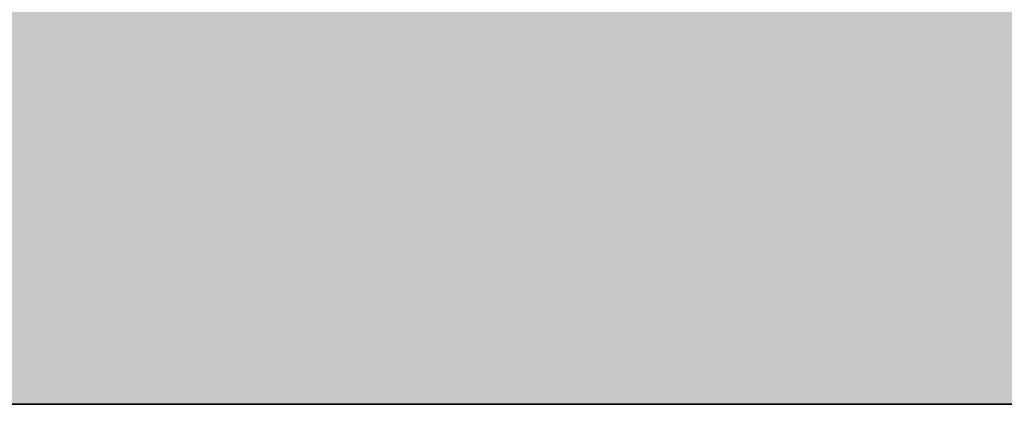
# Model space of a CAD drawing. Units: inches. Extents: x 2083 to 3317, y 1141 to 2115.
# Tile 143 of 256: x 3126.81755 to 3126.89136, y 1263.26136 to 1263.29018. Entities that reach past the tile are written whole.
import ezdxf

# ---------------------------------------------------------------- set-up
doc = ezdxf.new("R2010")
doc.units = ezdxf.units.IN
doc.layers.add('A-ANNO-DIMS', color=2, linetype='Continuous', lineweight=18)
doc.layers.add('A-WALL', color=7, linetype='Continuous', lineweight=35)
doc.layers.add('A-WALL-PATT', color=251, linetype='Continuous', lineweight=13, true_color=0x636466)
doc.styles.get("Standard").update_dxf_attribs({"font": 'arial.ttf'})
doc.dimstyles.new('ISO-25', dxfattribs={"dimtxt": 12, "dimasz": 12, "dimexe": 1.25, "dimexo": 0.625, "dimtad": 1, "dimlunit": 3, "dimtxsty": 'Standard', "dimcen": 2.5, "dimadec": 0, "dimazin": 0, "dimtfac": 1, "dimtmove": 0, "dimatfit": 3, "dimfxl": 1, "dimarcsym": 0})

# ---------------------------------------------------------------- blocks, each defined once
blk = doc.blocks.new('*D10')
at = {"layer": 'A-ANNO-DIMS', "color": 0, "lineweight": -2, "transparency": 16777216}
for p, q in [((2862.959783, 1262.63636), (2862.959783, 1201.38445)), ((3126.959783, 1262.63636), (3126.959783, 1201.38445)), ((2874.959783, 1202.63445), (3114.959783, 1202.63445))]:
    blk.add_line(p, q, dxfattribs=at)
at = {"layer": 'A-ANNO-DIMS', "color": 0, "transparency": 16777216}
for points in [[(2874.959783, 1204.63445), (2874.959783, 1200.63445), (2862.959783, 1202.63445)], [(3114.959783, 1204.63445), (3114.959783, 1200.63445), (3126.959783, 1202.63445)]]:
    blk.add_solid(points, dxfattribs=at)
at = {"layer": 'Defpoints', "color": 0, "transparency": 16777216}
for p in [(2862.959783, 1263.26136), (3126.959783, 1263.26136), (3126.959783, 1202.63445)]:
    blk.add_point(p, dxfattribs=at)
at = {"layer": 'A-ANNO-DIMS', "color": 0, "transparency": 16777216, "insert": (2994.959783, 1209.284006), "char_height": 12, "attachment_point": 5}
blk.add_mtext("22'", dxfattribs=at)
blk = doc.blocks.new('*D26')
at = {"layer": 'A-ANNO-DIMS', "color": 0, "lineweight": -2, "transparency": 16777216}
for p, q in [((3088.985844, 1274.915092), (3088.985844, 1270.951963)), ((3111.240037, 1274.915092), (3111.240037, 1270.951963)), ((3076.985844, 1272.201963), (2840.262447, 1272.201963)), ((3111.240037, 1272.201963), (3088.985844, 1272.201963)), ((3123.240037, 1272.201963), (3135.240037, 1272.201963))]:
    blk.add_line(p, q, dxfattribs=at)
at = {"layer": 'A-ANNO-DIMS', "color": 0, "transparency": 16777216}
for points in [[(3076.985844, 1274.201963), (3076.985844, 1270.201963), (3088.985844, 1272.201963)], [(3123.240037, 1274.201963), (3123.240037, 1270.201963), (3111.240037, 1272.201963)]]:
    blk.add_solid(points, dxfattribs=at)
at = {"layer": 'Defpoints', "color": 0, "transparency": 16777216}
for p in [(3088.985844, 1275.540092), (3111.240037, 1275.540092), (3088.985844, 1272.201963)]:
    blk.add_point(p, dxfattribs=at)
at = {"layer": 'A-ANNO-DIMS', "color": 0, "transparency": 16777216, "insert": (2952.624146, 1279.031602), "char_height": 12, "attachment_point": 5}
blk.add_mtext('NIGHTSTAND 1\'-10 1/2" TYP.', dxfattribs=at)
blk = doc.blocks.new('*D27')
at = {"layer": 'A-ANNO-DIMS', "color": 0, "lineweight": -2, "transparency": 16777216}
for p, q in [((3114.578165, 1309.794285), (3114.578165, 1321.794285)), ((3111.865037, 1297.794285), (3115.828165, 1297.794285)), ((3114.578165, 1297.794285), (3114.578165, 1275.540092)), ((3111.865037, 1275.540092), (3115.828165, 1275.540092)), ((3114.578165, 1263.540092), (3114.578165, 1140.988591))]:
    blk.add_line(p, q, dxfattribs=at)
at = {"layer": 'A-ANNO-DIMS', "color": 0, "transparency": 16777216}
for points in [[(3112.578165, 1309.794285), (3116.578165, 1309.794285), (3114.578165, 1297.794285)], [(3112.578165, 1263.540092), (3116.578165, 1263.540092), (3114.578165, 1275.540092)]]:
    blk.add_solid(points, dxfattribs=at)
at = {"layer": 'Defpoints', "color": 0, "transparency": 16777216}
for p in [(3111.240037, 1297.794285), (3111.240037, 1275.540092), (3114.578165, 1275.540092)]:
    blk.add_point(p, dxfattribs=at)
at = {"layer": 'A-ANNO-DIMS', "color": 0, "transparency": 16777216, "insert": (3107.748527, 1196.264342), "char_height": 12, "attachment_point": 5, "rotation": 90}
blk.add_mtext('1\'-10 1/2" TYP.', dxfattribs=at)

msp = doc.modelspace()

# ---------------------------------------------------------------- hatches: boundary and pattern name
at = {"layer": 'A-WALL-PATT'}
h = msp.add_hatch(color=256, dxfattribs=at)
h.dxf.hatch_style = 1
h.paths.add_polyline_path([(3126.959783, 2020.76136), (2748.959783, 2020.76136), (2604.959783, 2020.76136), (2226.959783, 2020.76136), (2226.959783, 1702.76136), (2466.959783, 1702.76136), (2466.959783, 1582.76136), (2418.959783, 1582.76136), (2418.959783, 1477.76136), (2226.959783, 1477.76136), (2226.959783, 1263.26136), (2544.959783, 1263.26136), (2544.959783, 1411.76136), (2604.959783, 1411.76136), (2685.959783, 1411.76136), (2685.959783, 1420.76136), (2604.959783, 1420.76136), (2604.959783, 1573.76136), (2604.959783, 1702.76136), (2604.959783, 2011.76136), (2748.959783, 2011.76136), (2748.959783, 1702.76136), (2862.959783, 1702.76136), (2862.959783, 1621.76136), (2871.959783, 1621.76136), (2871.959783, 1702.76136), (2883.959783, 1702.76136), (2883.959783, 1706.939459, -0.026459), (2883.959783, 1711.76136), (2757.959783, 1711.76136), (2757.959783, 1807.76136), (2787.959783, 1807.76136), (2787.959783, 1812.26136), (2757.959783, 1812.26136), (2757.959783, 2011.76136), (2877.959783, 2011.76136), (2877.959783, 1812.26136), (2847.959783, 1812.26136), (2847.959783, 1807.76136), (2889.835742, 1807.76136), (2889.835742, 1812.26136), (2882.459783, 1812.26136), (2882.459783, 2011.76136), (3117.959783, 2011.76136), (3117.959783, 1812.26136), (2937.835742, 1812.26136), (2937.835742, 1807.76136), (2995.709783, 1807.76136), (2995.709783, 1796.117666), (3000.209783, 1796.117666), (3000.209783, 1807.76136), (3117.959783, 1807.76136), (3117.959783, 1711.76136), (3000.209783, 1711.76136), (3000.209783, 1760.117666), (2998.572705, 1760.117666, -0.020711), (2995.709783, 1760.117666), (2995.709783, 1711.76136), (2931.959783, 1711.76136), (2931.959783, 1702.76136), (3126.959783, 1702.76136)])
h.paths.add_polyline_path([(2471.459783, 2011.76136), (2471.459783, 1810.01136), (2462.716936, 1810.01136), (2462.716936, 1805.51136), (2505.959783, 1805.51136), (2505.959783, 1810.01136), (2475.959783, 1810.01136), (2475.959783, 2011.76136), (2595.959783, 2011.76136), (2595.959783, 1810.01136), (2565.959783, 1810.01136), (2565.959783, 1805.51136), (2595.959783, 1805.51136), (2595.959783, 1711.76136), (2235.959783, 1711.76136), (2235.959783, 1805.51136), (2353.709783, 1805.51136), (2353.709783, 1796.054162), (2358.209783, 1796.054162), (2358.209783, 1805.51136), (2414.716936, 1805.51136), (2414.716936, 1810.01136), (2235.959783, 1810.01136), (2235.959783, 2011.76136)], flags=16)
h.paths.add_polyline_path([(2270.204734, 1994.610008), (2270.204734, 1970.610008), (2246.204734, 1970.610008), (2246.204734, 1994.610008)], flags=0)
edge = h.paths.add_edge_path(flags=0)
edge.add_ellipse((2332.027391, 1899.798176), major_axis=(-3.042994, 3.042994), ratio=0.16825245, start_angle=-161.332166, end_angle=-156.307114, ccw=False)
edge.add_ellipse((2333.082037, 1898.74353), major_axis=(-1.054646, 1.054646), ratio=0.4535321, start_angle=-123.371019, end_angle=-94.159107)
edge = h.paths.add_edge_path(flags=0)
edge.add_ellipse((2332.027391, 1968.87629), major_axis=(3.042994, 3.042994), ratio=0.16825245, start_angle=18.667834, end_angle=23.692886)
edge.add_spline(control_points=[(2332.925596, 1970.691105), (2332.226768, 1970.3361), (2330.893709, 1969.658905), (2328.41308, 1970.932138), (2327.203934, 1967.748712), (2324.709596, 1969.955589), (2322.532822, 1967.012354), (2320.012846, 1971.295812), (2317.680308, 1968.157845), (2316.040526, 1967.102047), (2315.426904, 1966.809602)], knot_values=[0, 0, 0, 0, 2.267059, 4.324559, 6.685584, 8.878641, 11.121502, 14.300359, 17.755284, 19.732645, 19.732645, 19.732645, 19.732645], degree=3, periodic=0)
edge.add_ellipse((2332.027391, 1968.87629), major_axis=(3.042994, 3.042994), ratio=0.16825245, start_angle=18.667834, end_angle=23.692886, ccw=False)
edge.add_ellipse((2333.082037, 1969.930936), major_axis=(1.054646, 1.054646), ratio=0.4535321, start_angle=56.628981, end_angle=85.840893, ccw=False)
edge = h.paths.add_edge_path(flags=0)
edge.add_spline(control_points=[(2296.428287, 1967.987908), (2293.627804, 1965.336314), (2287.703624, 1959.727094), (2299.74386, 1949.995699), (2294.532591, 1935.668528), (2290.573228, 1920.603512), (2293.394124, 1909.973691), (2296.185407, 1904.966543)], knot_values=[0.099185, 0.099185, 0.099185, 0.099185, 0.345301, 0.619822, 0.982653, 1.386093, 1.810555, 1.810555, 1.810555, 1.810555], degree=3, periodic=0)
edge.add_spline(control_points=[(2296.185407, 1904.966543), (2297.383582, 1902.6193), (2298.000969, 1901.949312), (2298.55297, 1901.468155)], knot_values=[0.006246, 0.006246, 0.006246, 0.006246, 0.055476, 0.055476, 0.055476, 0.055476], degree=3, periodic=0)
edge.add_spline(control_points=[(2298.55297, 1901.468155), (2297.258612, 1900.923224), (2295.225294, 1900.232126), (2293.060229, 1900.614205), (2292.101423, 1900.788415), (2292.089578, 1900.790568)], knot_values=[0.312835, 0.312835, 0.312835, 0.312835, 0.40178, 0.474987, 0.475903, 0.475903, 0.475903, 0.475903], degree=3, periodic=0)
edge.add_arc((2292.793646, 1904.664109), 3.937008, 215.420897, 259.698179, ccw=False)
edge.add_spline(control_points=[(2289.585314, 1902.382304), (2289.476652, 1902.535087), (2289.36848, 1902.688035), (2289.260865, 1902.84117)], knot_values=[0.102872, 0.102872, 0.102872, 0.102872, 0.116896, 0.116896, 0.116896, 0.116896], degree=3, periodic=0)
edge.add_spline(control_points=[(2289.260865, 1902.84117), (2288.686604, 1902.550192), (2287.640048, 1902.019902), (2285.881337, 1901.873954), (2283.852972, 1901.504352), (2281.719987, 1899.710538), (2278.466991, 1899.492942), (2276.157136, 1901.883202), (2272.258953, 1899.804071), (2267.777605, 1901.843183), (2262.243882, 1900.184033), (2257.414927, 1901.782061), (2254.318374, 1900.72612), (2253.178285, 1900.337343)], knot_values=[0, 0, 0, 0, 1.907977, 3.477176, 5.261074, 7.972851, 11.680248, 13.717921, 16.939592, 22.789562, 27.502503, 33.595215, 37.145618, 37.145618, 37.145618, 37.145618], degree=3, periodic=0)
edge.add_line((2253.178285, 1900.337343), (2250.24424, 1902.84117))
edge.add_line((2250.24424, 1902.84117), (2250.24424, 1965.833296))
edge.add_line((2250.24424, 1965.833296), (2253.178285, 1968.337123))
edge.add_spline(control_points=[(2253.178285, 1968.337123), (2254.318374, 1967.948346), (2257.414927, 1966.892405), (2262.243882, 1968.490433), (2267.777605, 1966.831283), (2271.52673, 1968.537217), (2273.875914, 1967.828289), (2274.206701, 1967.727642)], knot_values=[0, 0, 0, 0, 0.09018, 0.244935, 0.364644, 0.513233, 0.537855, 0.537855, 0.537855, 0.537855], degree=3, periodic=0)
edge.add_arc((2274.352887, 1963.793349), 3.937008, 72.051134, 92.127949, ccw=False)
edge.add_arc((2281.296933, 1985.230003), 18.596298, 252.0511336, 288.5657217)
edge.add_arc((2292.316717, 1956.02888), 12.646081, 71.0267879, 113.7782184, ccw=False)
edge = h.paths.add_edge_path(flags=0)
edge.add_spline(control_points=[(2274.899415, 1951.856195), (2275.066156, 1951.616592), (2275.232687, 1951.376588), (2275.397987, 1951.135855)], knot_values=[1.409916, 1.409916, 1.409916, 1.409916, 1.43159, 1.43159, 1.43159, 1.43159], degree=3, periodic=0)
edge.add_spline(control_points=[(2275.397987, 1951.135855), (2275.792106, 1950.561885), (2276.179231, 1949.983774), (2276.545546, 1949.397103)], knot_values=[1.358238, 1.358238, 1.358238, 1.358238, 1.409916, 1.409916, 1.409916, 1.409916], degree=3, periodic=0)
edge.add_line((2276.545546, 1949.397103), (2277.437289, 1947.862185))
edge.add_spline(control_points=[(2277.437289, 1947.862185), (2276.303834, 1945.673115), (2274.639698, 1942.426882), (2274.631615, 1938.0939), (2272.799124, 1930.85155), (2274.356426, 1943.897046), (2275.947681, 1947.923356), (2276.545546, 1949.397103)], knot_values=[0.005632, 0.005632, 0.005632, 0.005632, 0.186014, 0.266002, 0.357087, 0.59639, 0.739732, 0.739732, 0.739732, 0.739732], degree=3, periodic=0)
edge.add_spline(control_points=[(2276.545546, 1949.397103), (2276.179231, 1949.983774), (2275.792106, 1950.561885), (2275.397987, 1951.135855)], knot_values=[1.358238, 1.358238, 1.358238, 1.358238, 1.409916, 1.409916, 1.409916, 1.409916], degree=3, periodic=0)
edge.add_spline(control_points=[(2275.397987, 1951.135855), (2274.9425, 1950.080452), (2274.20776, 1948.025272), (2273.934602, 1944.851477), (2272.468534, 1937.627489), (2273.466216, 1945.696466), (2274.700615, 1951.059472), (2274.899415, 1951.856195)], knot_values=[0.104364, 0.104364, 0.104364, 0.104364, 0.189636, 0.269624, 0.36071, 0.600013, 0.644622, 0.644622, 0.644622, 0.644622], degree=3, periodic=0)
h.paths.add_polyline_path([(2269.167514, 1963.127573, -0.357527), (2268.170633, 1960.97637, -0.092561), (2268.170633, 1939.436325, -0.357527), (2269.167514, 1937.285122, -0.357527), (2267.01631, 1938.282002, -0.164785), (2254.685581, 1938.282002, -0.357527), (2252.534378, 1937.285122, -0.357527), (2253.531259, 1939.436325, -0.092561), (2253.531259, 1960.97637, -0.357527), (2252.534378, 1963.127573, -0.357527), (2254.685581, 1962.130692, -0.164785), (2267.01631, 1962.130692, -0.357527)], flags=0)
h.paths.add_polyline_path([(2248.874068, 1967.8018), (2248.874068, 1957.02771), (2249.457783, 1957.02771), (2249.457783, 1911.646756), (2248.874068, 1911.646756), (2248.874068, 1900.872666), (2246.511863, 1900.872666, 0.197327), (2244.149658, 1902.456873), (2244.149658, 1966.217592, 0.197327), (2246.511863, 1967.8018)], flags=0)
h.paths.add_polyline_path([(2269.167514, 1931.389344, -0.357527), (2268.170633, 1929.238141, -0.092561), (2268.170633, 1907.698096, -0.357527), (2269.167514, 1905.546893, -0.357527), (2267.01631, 1906.543774, -0.164785), (2254.685581, 1906.543774, -0.357527), (2252.534378, 1905.546893, -0.357527), (2253.531259, 1907.698096, -0.092561), (2253.531259, 1929.238141, -0.357527), (2252.534378, 1931.389344, -0.357527), (2254.685581, 1930.392463, -0.164785), (2267.01631, 1930.392463, -0.357527)], flags=0)
edge = h.paths.add_edge_path(flags=0)
edge.add_spline(control_points=[(2276.196858, 1906.723702), (2276.168144, 1909.028928), (2276.114049, 1913.371852), (2270.598417, 1924.924978), (2273.905175, 1919.012779), (2275.921711, 1916.262063), (2275.47457, 1912.402149), (2277.257874, 1910.380621), (2276.696044, 1908.225036), (2276.646218, 1906.813023), (2276.617825, 1906.008407)], knot_values=[0, 0, 0, 0, 8.61026, 16.221274, 18.843057, 23.804898, 27.440828, 29.356102, 31.203478, 33.650687, 33.650687, 33.650687, 33.650687], degree=3, periodic=0)
edge.add_spline(control_points=[(2276.617825, 1906.008407), (2276.623313, 1905.624144), (2276.497738, 1904.628661), (2275.441779, 1903.854725), (2274.937314, 1903.08045), (2274.85908, 1902.84117)], knot_values=[0.156488, 0.156488, 0.156488, 0.156488, 0.184398, 0.231376, 0.250598, 0.250598, 0.250598, 0.250598], degree=3, periodic=0)
edge.add_line((2274.85908, 1902.84117), (2276.50598, 1902.84117))
edge.add_spline(control_points=[(2276.50598, 1902.84117), (2276.788308, 1903.08494), (2277.665071, 1904.125196), (2278.249538, 1904.340738), (2277.653872, 1908.527387), (2278.15567, 1906.227808), (2278.100464, 1905.285948), (2278.846675, 1904.069005), (2277.856785, 1903.414948), (2277.874191, 1902.99105), (2277.903562, 1902.84117)], knot_values=[0.059574, 0.059574, 0.059574, 0.059574, 0.080753, 0.103741, 0.16972, 0.176036, 0.207137, 0.240474, 0.262341, 0.27366, 0.27366, 0.27366, 0.27366], degree=3, periodic=0)
edge.add_line((2277.903562, 1902.84117), (2280.029825, 1902.84117))
edge.add_spline(control_points=[(2280.029825, 1902.84117), (2279.888221, 1903.088398), (2279.499257, 1903.981551), (2280.152284, 1905.939349), (2278.103615, 1909.657757), (2279.762395, 1907.185285), (2280.3279, 1904.874861), (2280.485109, 1903.48959), (2281.463269, 1903.249432), (2281.758343, 1902.936497), (2281.834036, 1902.84117)], knot_values=[0.013856, 0.013856, 0.013856, 0.013856, 0.034874, 0.088867, 0.107879, 0.126738, 0.158714, 0.193757, 0.217487, 0.226722, 0.226722, 0.226722, 0.226722], degree=3, periodic=0)
edge.add_spline(control_points=[(2281.834036, 1902.84117), (2281.787535, 1902.826703), (2281.647022, 1902.782988), (2281.395527, 1902.85949), (2281.088077, 1902.985242), (2280.720683, 1903.060902), (2280.333451, 1903.025726), (2280.124767, 1902.898879), (2280.029825, 1902.84117)], knot_values=[0, 0, 0, 0, 0.14413, 0.435517, 0.749276, 1.153046, 1.548371, 1.878348, 1.878348, 1.878348, 1.878348], degree=3, periodic=0)
edge.add_line((2280.029825, 1902.84117), (2277.903562, 1902.84117))
edge.add_spline(control_points=[(2277.903562, 1902.84117), (2277.892855, 1902.795855), (2277.865396, 1902.679637), (2277.607479, 1902.687483), (2277.27405, 1902.8007), (2276.837921, 1902.619775), (2276.583807, 1902.789261), (2276.50598, 1902.84117)], knot_values=[0, 0, 0, 0, 0.127189, 0.326199, 0.628009, 1.24357, 1.515331, 1.515331, 1.515331, 1.515331], degree=3, periodic=0)
edge.add_line((2276.50598, 1902.84117), (2274.85908, 1902.84117))
edge.add_spline(control_points=[(2274.85908, 1902.84117), (2274.814437, 1902.898587), (2274.72513, 1903.013446), (2274.493477, 1903.118968), (2274.244285, 1902.960539), (2273.937121, 1903.184942), (2273.614039, 1902.983143), (2273.408316, 1902.883045), (2273.322254, 1902.84117)], knot_values=[0, 0, 0, 0, 0.21843, 0.436957, 0.687977, 0.990379, 1.398396, 1.69185, 1.69185, 1.69185, 1.69185], degree=3, periodic=0)
edge.add_spline(control_points=[(2273.322254, 1902.84117), (2273.61674, 1903.445692), (2274.273998, 1904.538253), (2276.027239, 1904.573702), (2276.206963, 1906.583637), (2276.196858, 1906.723702)], knot_values=[0.012227, 0.012227, 0.012227, 0.012227, 0.059472, 0.106218, 0.134458, 0.134458, 0.134458, 0.134458], degree=3, periodic=0)
h.paths.add_polyline_path([(2270.776054, 1897.789828), (2270.776054, 1873.789828), (2246.776054, 1873.789828), (2246.776054, 1897.789828)], flags=0)
h.paths.add_polyline_path([(2353.709783, 1760.005059), (2353.709783, 1760.054162), (2358.209783, 1760.054162, -0.033729)], flags=0)
h.paths.add_polyline_path([(2321.819119, 1737.529186), (2341.995327, 1737.529186, -0.414214), (2343.203273, 1736.321241), (2343.203273, 1721.020596, -0.414214), (2341.995327, 1719.812651), (2321.819119, 1719.812651, -0.414214), (2320.611173, 1721.020596), (2320.611173, 1736.321241, -0.414214)], flags=0)
h.paths.add_polyline_path([(2324.23501, 1736.321241), (2339.579436, 1736.321241, -0.414214), (2341.995327, 1733.905349), (2341.995327, 1725.44973, -0.414214), (2339.579436, 1723.033839), (2333.680588, 1723.033839), (2333.845317, 1722.045467, -0.870646), (2335.425399, 1721.825893, -0.767327), (2333.922694, 1721.423245), (2331.291024, 1721.423245, -0.767327), (2329.788319, 1721.825893, -0.870646), (2331.368401, 1722.045467), (2331.53313, 1723.033839), (2324.23501, 1723.033839, -0.414214), (2321.819119, 1725.44973), (2321.819119, 1733.905349, -0.414214)], flags=0)
h.paths.add_polyline_path([(2570.483789, 1928.615444), (2589.683789, 1928.615444), (2590.168829, 1928.615444), (2590.168829, 1904.993397), (2570.483789, 1904.993397)], flags=0)
h.paths.add_polyline_path([(2574.447324, 1927.263822, -1), (2572.828836, 1927.263822, -1)], flags=0)
h.paths.add_polyline_path([(2573.089867, 1926.940877), (2573.925032, 1927.776042), (2574.147743, 1927.553332), (2573.312577, 1926.718166)], flags=0)
h.paths.add_polyline_path([(2578.779065, 1919.729618, -1), (2571.591663, 1919.729618, -1)], flags=0)
h.paths.add_polyline_path([(2578.385364, 1919.729618, -1), (2571.985364, 1919.729618, -1)], flags=0)
h.paths.add_polyline_path([(2331.595764, 1729.476216, -1), (2333.617954, 1729.476216, -1)], flags=0)
h.paths.add_polyline_path([(2578.034228, 1927.263822, -1), (2576.41574, 1927.263822, -1)], flags=0)
h.paths.add_polyline_path([(2576.688851, 1927.531089), (2576.911562, 1927.753799), (2577.746728, 1926.918634), (2577.524017, 1926.695923)], flags=0)
h.paths.add_polyline_path([(2578.139065, 1909.859539, -1), (2572.231663, 1909.859539, -1)], flags=0)
h.paths.add_polyline_path([(2577.745364, 1909.859539, -1), (2572.625364, 1909.859539, -1)], flags=0)
h.paths.add_polyline_path([(2583.797718, 1927.263822, -1), (2582.179229, 1927.263822, -1)], flags=0)
h.paths.add_polyline_path([(2582.718649, 1927.753799), (2583.553814, 1926.918634), (2583.331103, 1926.695923), (2582.495938, 1927.531089)], flags=0)
h.paths.add_polyline_path([(2582.495938, 1927.531089), (2582.718649, 1927.753799), (2583.553814, 1926.918634), (2583.331103, 1926.695923)], flags=0)
h.paths.add_polyline_path([(2587.739065, 1920.529618, -1), (2581.831663, 1920.529618, -1)], flags=0)
h.paths.add_polyline_path([(2587.345364, 1920.529618, -1), (2582.225364, 1920.529618, -1)], flags=0)
h.paths.add_polyline_path([(2587.384622, 1927.263822, -1), (2585.766133, 1927.263822, -1)], flags=0)
h.paths.add_polyline_path([(2586.081993, 1926.980247), (2586.917158, 1927.815412), (2587.139869, 1927.592702), (2586.304703, 1926.757536)], flags=0)
h.paths.add_polyline_path([(2588.379065, 1910.659539, -1), (2581.191663, 1910.659539, -1)], flags=0)
h.paths.add_polyline_path([(2587.985364, 1910.659539, -1), (2581.585364, 1910.659539, -1)], flags=0)
h.paths.add_polyline_path([(2417.167729, 1729.477895), (2437.343937, 1729.477895, -0.414214), (2438.551883, 1728.26995), (2438.551883, 1712.969306, -0.414214), (2437.343937, 1711.76136), (2417.167729, 1711.76136, -0.414214), (2415.959783, 1712.969306), (2415.959783, 1728.26995, -0.414214)], flags=0)
h.paths.add_polyline_path([(2419.58362, 1728.26995), (2434.928046, 1728.26995, -0.414214), (2437.343937, 1725.854059), (2437.343937, 1717.39844, -0.414214), (2434.928046, 1714.982548), (2429.029199, 1714.982548), (2429.193927, 1713.994176, -0.870646), (2430.774009, 1713.774603, -0.767327), (2429.271304, 1713.371954), (2426.639634, 1713.371954, -0.767327), (2425.136929, 1713.774603, -0.870646), (2426.717011, 1713.994176), (2426.88174, 1714.982548), (2419.58362, 1714.982548, -0.414214), (2417.167729, 1717.39844), (2417.167729, 1725.854059, -0.414214)], flags=0)
h.paths.add_polyline_path([(2419.58362, 1728.26995), (2434.928046, 1728.26995, -0.414214), (2437.343937, 1725.854059), (2437.343937, 1717.39844, -0.414214), (2434.928046, 1714.982548), (2429.029199, 1714.982548), (2428.358118, 1719.009034), (2427.552821, 1719.009034), (2426.88174, 1714.982548), (2419.58362, 1714.982548, -0.414214), (2417.167729, 1717.39844), (2417.167729, 1725.854059, -0.414214)], flags=0)
h.paths.add_polyline_path([(2426.944374, 1721.424925, -1), (2428.966564, 1721.424925, -1)], flags=0)
h.paths.add_polyline_path([(2475.959783, 1702.76136), (2595.959783, 1702.76136), (2595.959783, 1582.76136), (2475.959783, 1582.76136)], flags=16)
h.paths.add_polyline_path([(2427.959783, 1573.76136), (2595.959783, 1573.76136), (2595.959783, 1468.76136), (2595.959783, 1420.76136), (2384.459783, 1420.76136), (2384.459783, 1468.76136), (2427.959783, 1468.76136)], flags=16)
h.paths.add_polyline_path([(2379.959783, 1468.76136), (2379.959783, 1420.76136), (2235.959783, 1420.76136), (2235.959783, 1468.76136)], flags=16)
h.paths.add_polyline_path([(2317.815996, 1466.695767), (2337.992205, 1466.695767, -0.414214), (2339.20015, 1465.487821), (2339.20015, 1450.187177, -0.414214), (2337.992205, 1448.979232), (2317.815996, 1448.979232, -0.414214), (2316.608051, 1450.187177), (2316.608051, 1465.487821, -0.414214)], flags=0)
h.paths.add_polyline_path([(2320.231887, 1465.487821), (2335.576313, 1465.487821, -0.414214), (2337.992205, 1463.07193), (2337.992205, 1454.616311, -0.414214), (2335.576313, 1452.20042), (2329.677466, 1452.20042), (2329.842195, 1451.212047, -0.870646), (2331.422276, 1450.992474, -0.767327), (2329.919571, 1450.589826), (2327.287902, 1450.589826, -0.767327), (2325.785197, 1450.992474, -0.870646), (2327.365278, 1451.212047), (2327.530007, 1452.20042), (2320.231887, 1452.20042, -0.414214), (2317.815996, 1454.616311), (2317.815996, 1463.07193, -0.414214)], flags=0)
h.paths.add_polyline_path([(2320.231887, 1465.487821), (2335.576313, 1465.487821, -0.414214), (2337.992205, 1463.07193), (2337.992205, 1454.616311, -0.414214), (2335.576313, 1452.20042), (2329.677466, 1452.20042), (2329.006385, 1456.226905), (2328.201088, 1456.226905), (2327.530007, 1452.20042), (2320.231887, 1452.20042, -0.414214), (2317.815996, 1454.616311), (2317.815996, 1463.07193, -0.414214)], flags=0)
h.paths.add_polyline_path([(2327.592641, 1458.642796, -1), (2329.614832, 1458.642796, -1)], flags=0)
h.paths.add_polyline_path([(2244.411744, 1433.340453), (2241.920945, 1433.340453, -0.414214), (2240.017856, 1435.243542), (2240.017856, 1440.952808, -0.414211), (2241.920925, 1442.855897), (2244.411744, 1442.855897, -1.976472)], flags=0)
h.paths.add_polyline_path([(2245.356888, 1434.397536, -0.414214), (2245.356888, 1441.798814, -2.144098)], flags=0)
h.paths.add_polyline_path([(2535.959783, 1416.26136), (2535.959783, 1272.26136), (2235.959783, 1272.26136), (2235.959783, 1416.26136)], flags=16)
h.paths.add_polyline_path([(2260.119561, 1384.292841), (2260.119561, 1362.038649), (2237.865369, 1362.038649), (2237.865369, 1384.292841)], flags=0)
edge = h.paths.add_edge_path(flags=0)
edge.add_line((2318.251847, 1362.093298), (2318.145797, 1362.000973))
edge.add_ellipse((2317.445116, 1360.431044), major_axis=(2.82164, 2.82164), ratio=0.16825245, start_angle=18.667834, end_angle=20.948127, ccw=False)
edge.add_ellipse((2318.423045, 1361.408974), major_axis=(0.977929, 0.977929), ratio=0.4535321, start_angle=56.628981, end_angle=70.226201, ccw=False)
edge = h.paths.add_edge_path(flags=0)
edge.add_line((2319.10737, 1295.571078), (2319.015044, 1295.677128))
edge.add_ellipse((2317.445116, 1296.377809), major_axis=(-2.82164, 2.82164), ratio=0.16825245, start_angle=-161.332166, end_angle=-159.051873, ccw=False)
edge.add_ellipse((2318.423045, 1295.39988), major_axis=(-0.977929, 0.977929), ratio=0.4535321, start_angle=-123.371019, end_angle=-109.773799)
edge = h.paths.add_edge_path(flags=0)
edge.add_spline(control_points=[(2284.210349, 1301.170219), (2284.580688, 1300.444719), (2284.891189, 1299.892024), (2285.159553, 1299.461018)], knot_values=[0.039066, 0.039066, 0.039066, 0.039066, 0.055476, 0.055476, 0.055476, 0.055476], degree=3, periodic=0)
edge.add_line((2285.159553, 1299.461018), (2284.210349, 1301.170219))
edge = h.paths.add_edge_path(flags=0)
edge.add_line((2280.412458, 1297.298013), (2283.369991, 1297.036122))
edge.add_line((2283.369991, 1297.036122), (2286.40569, 1297.92631))
edge.add_spline(control_points=[(2286.40569, 1297.92631), (2285.305487, 1297.463119), (2284.344777, 1297.129151), (2283.369991, 1297.036122)], knot_values=[0.394369, 0.394369, 0.394369, 0.394369, 0.475903, 0.475903, 0.475903, 0.475903], degree=3, periodic=0)
edge.add_spline(control_points=[(2283.369991, 1297.036122), (2283.28139, 1297.027666), (2282.316289, 1296.957336), (2281.312502, 1297.134479), (2280.423441, 1297.296016), (2280.412458, 1297.298013)], knot_values=[0.312835, 0.312835, 0.312835, 0.312835, 0.320246, 0.393453, 0.394369, 0.394369, 0.394369, 0.394369], degree=3, periodic=0)
edge = h.paths.add_edge_path(flags=0)
edge.add_line((2284.435561, 1359.607285), (2280.446291, 1355.328047))
edge.add_line((2280.446291, 1355.328047), (2279.579987, 1351.017754))
edge.add_line((2279.579987, 1351.017754), (2282.412974, 1346.580433))
edge.add_spline(control_points=[(2282.412974, 1346.580433), (2283.153331, 1345.589236), (2284.252896, 1344.028897), (2284.801037, 1342.387167), (2284.935162, 1341.805544)], knot_values=[1.240098, 1.240098, 1.240098, 1.240098, 1.332892, 1.382712, 1.382712, 1.382712, 1.382712], degree=3, periodic=0)
edge.add_spline(control_points=[(2284.935162, 1341.805544), (2285.319108, 1340.1406), (2285.233029, 1338.409204), (2284.909938, 1336.654122)], knot_values=[1.097484, 1.097484, 1.097484, 1.097484, 1.240098, 1.240098, 1.240098, 1.240098], degree=3, periodic=0)
edge.add_spline(control_points=[(2284.909938, 1336.654122), (2284.586848, 1334.89904), (2284.026745, 1333.120272), (2283.462644, 1331.360585)], knot_values=[0.95487, 0.95487, 0.95487, 0.95487, 1.097484, 1.097484, 1.097484, 1.097484], degree=3, periodic=0)
edge.add_line((2283.462644, 1331.360585), (2281.890376, 1326.153357))
edge.add_line((2281.890376, 1326.153357), (2280.756259, 1321.056089))
edge.add_line((2280.756259, 1321.056089), (2280.299205, 1316.001977))
edge.add_line((2280.299205, 1316.001977), (2280.715933, 1310.950068))
edge.add_line((2280.715933, 1310.950068), (2282.028094, 1305.972137))
edge.add_line((2282.028094, 1305.972137), (2284.210349, 1301.170219))
edge.add_spline(control_points=[(2284.210349, 1301.170219), (2283.340731, 1302.730185), (2282.611904, 1304.336493), (2282.028094, 1305.972137)], knot_values=[0.099185, 0.099185, 0.099185, 0.099185, 0.241799, 0.241799, 0.241799, 0.241799], degree=3, periodic=0)
edge.add_spline(control_points=[(2282.028094, 1305.972137), (2281.444283, 1307.60778), (2281.005489, 1309.272759), (2280.715933, 1310.950068)], knot_values=[0.241799, 0.241799, 0.241799, 0.241799, 0.384413, 0.384413, 0.384413, 0.384413], degree=3, periodic=0)
edge.add_spline(control_points=[(2280.715933, 1310.950068), (2280.433241, 1312.587613), (2280.289386, 1314.276959), (2280.298894, 1315.962032), (2280.299205, 1316.001977)], knot_values=[0.384413, 0.384413, 0.384413, 0.384413, 0.523647, 0.527028, 0.527028, 0.527028, 0.527028], degree=3, periodic=0)
edge.add_spline(control_points=[(2280.299205, 1316.001977), (2280.312326, 1317.686955), (2280.477871, 1319.367926), (2280.756259, 1321.056089)], knot_values=[0.527028, 0.527028, 0.527028, 0.527028, 0.669642, 0.669642, 0.669642, 0.669642], degree=3, periodic=0)
edge.add_spline(control_points=[(2280.756259, 1321.056089), (2281.034648, 1322.744252), (2281.42588, 1324.439608), (2281.890376, 1326.153357)], knot_values=[0.669642, 0.669642, 0.669642, 0.669642, 0.812256, 0.812256, 0.812256, 0.812256], degree=3, periodic=0)
edge.add_spline(control_points=[(2281.890376, 1326.153357), (2282.264383, 1327.533251), (2282.78787, 1329.26181), (2283.352751, 1331.01778), (2283.462644, 1331.360585)], knot_values=[0.812256, 0.812256, 0.812256, 0.812256, 0.927087, 0.95487, 0.95487, 0.95487, 0.95487], degree=3, periodic=0)
edge.add_line((2283.462644, 1331.360585), (2284.909938, 1336.654122))
edge.add_line((2284.909938, 1336.654122), (2284.935162, 1341.805544))
edge.add_line((2284.935162, 1341.805544), (2282.412974, 1346.580433))
edge.add_spline(control_points=[(2282.412974, 1346.580433), (2281.275127, 1348.103792), (2280.078447, 1349.570318), (2279.579987, 1351.017754)], knot_values=[1.382712, 1.382712, 1.382712, 1.382712, 1.525326, 1.525326, 1.525326, 1.525326], degree=3, periodic=0)
edge.add_spline(control_points=[(2279.579987, 1351.017754), (2279.443282, 1351.414721), (2279.136312, 1352.856922), (2279.73519, 1354.290385), (2280.446291, 1355.328047)], knot_values=[1.525326, 1.525326, 1.525326, 1.525326, 1.564439, 1.667941, 1.667941, 1.667941, 1.667941], degree=3, periodic=0)
edge.add_spline(control_points=[(2280.446291, 1355.328047), (2281.426113, 1356.757835), (2282.930837, 1358.18256), (2284.435561, 1359.607285)], knot_values=[1.667941, 1.667941, 1.667941, 1.667941, 1.810555, 1.810555, 1.810555, 1.810555], degree=3, periodic=0)
edge.add_arc((2280.623075, 1348.518181), 11.72618, 71.0267879, 113.7782184)
edge.add_arc((2270.404892, 1375.595156), 17.243567, 252.0511336, 288.5657217, ccw=False)
edge.add_arc((2263.965969, 1355.717847), 3.650622, 72.051134, 92.127949)
edge.add_arc((2263.965969, 1355.717847), 3.650622, 92.127949, 177.98513)
edge.add_spline(control_points=[(2260.317604, 1355.846199), (2260.260417, 1354.220668), (2260.551278, 1350.186547), (2262.999344, 1346.766251), (2264.472741, 1344.649024)], knot_values=[1.43159, 1.43159, 1.43159, 1.43159, 1.564144, 1.770695, 1.770695, 1.770695, 1.770695], degree=3, periodic=0)
edge.add_line((2264.472741, 1344.649024), (2264.93559, 1343.98253))
edge.add_spline(control_points=[(2263.801044, 1340.248105), (2263.843238, 1340.514088), (2264.067244, 1341.756465), (2264.512693, 1343.002453), (2264.935047, 1343.981083)], knot_values=[0.53657, 0.53657, 0.53657, 0.53657, 0.559349, 0.644622, 0.644622, 0.644622, 0.644622], degree=3, periodic=0)
edge.add_spline(control_points=[(2264.935047, 1343.981083), (2265.117771, 1343.714975), (2265.298875, 1343.447906), (2265.476756, 1343.179365)], knot_values=[1.384077, 1.384077, 1.384077, 1.384077, 1.409916, 1.409916, 1.409916, 1.409916], degree=3, periodic=0)
edge.add_spline(control_points=[(2265.476756, 1343.179365), (2265.654637, 1342.910823), (2265.829296, 1342.64081), (2265.99913, 1342.368812)], knot_values=[1.358238, 1.358238, 1.358238, 1.358238, 1.384077, 1.384077, 1.384077, 1.384077], degree=3, periodic=0)
edge.add_line((2265.99913, 1342.368812), (2266.826006, 1340.945547))
edge.add_spline(control_points=[(2266.826006, 1340.945547), (2268.894401, 1337.089691), (2271.398173, 1325.843001), (2270.516164, 1310.568557), (2275.919376, 1301.860609), (2277.789511, 1299.19945)], knot_values=[0.116896, 0.116896, 0.116896, 0.116896, 0.472987, 1.050969, 1.313793, 1.313793, 1.313793, 1.313793], degree=3, periodic=0)
edge.add_spline(control_points=[(2277.789511, 1299.19945), (2277.839405, 1299.128452), (2277.889428, 1299.057498), (2277.939572, 1298.986584)], knot_values=[0.109884, 0.109884, 0.109884, 0.109884, 0.116896, 0.116896, 0.116896, 0.116896], degree=3, periodic=0)
edge.add_line((2277.939572, 1298.986584), (2277.788849, 1299.199114))
edge.add_spline(control_points=[(2277.788849, 1299.199114), (2277.256582, 1298.929414), (2276.28635, 1298.437902), (2275.039352, 1298.334419), (2274.38333, 1298.238895), (2274.215254, 1298.209338)], knot_values=[33.12187, 33.12187, 33.12187, 33.12187, 35.029056, 36.598255, 37.144827, 37.144827, 37.144827, 37.144827], degree=3, periodic=0)
edge.add_line((2274.215254, 1298.209338), (2273.073147, 1297.892961))
edge.add_spline(control_points=[(2273.073147, 1297.892961), (2272.322936, 1297.579784), (2271.039151, 1296.510508), (2269.248395, 1296.226062), (2268.4231, 1296.374654)], knot_values=[26.532584, 26.532584, 26.532584, 26.532584, 29.198919, 31.839101, 31.839101, 31.839101, 31.839101], degree=3, periodic=0)
edge.add_line((2268.4231, 1296.374654), (2263.878501, 1297.457534))
edge.add_spline(control_points=[(2263.878501, 1297.457534), (2263.556077, 1297.359435), (2261.860306, 1296.838694), (2260.23878, 1297.282407), (2258.933454, 1297.516461)], knot_values=[15.919551, 15.919551, 15.919551, 15.919551, 16.939592, 21.226067, 21.226067, 21.226067, 21.226067], degree=3, periodic=0)
edge.add_line((2258.933454, 1297.516461), (2254.055233, 1297.32901))
edge.add_spline(control_points=[(2254.055233, 1297.32901), (2253.755525, 1297.295815), (2252.113683, 1297.165174), (2250.461869, 1297.544221), (2249.129686, 1297.667882)], knot_values=[5.306517, 5.306517, 5.306517, 5.306517, 6.276435, 10.613034, 10.613034, 10.613034, 10.613034], degree=3, periodic=0)
edge.add_line((2249.129686, 1297.667882), (2244.33165, 1296.877756))
edge.add_line((2244.33165, 1296.877756), (2241.611033, 1299.19945))
edge.add_line((2241.611033, 1299.19945), (2241.611033, 1357.609404))
edge.add_line((2241.611033, 1357.609404), (2244.33165, 1359.931097))
edge.add_line((2244.33165, 1359.931097), (2252.728823, 1359.542692))
edge.add_spline(control_points=[(2252.728823, 1359.542692), (2252.870939, 1359.54644), (2253.30574, 1359.548172), (2253.739845, 1359.514274), (2254.031742, 1359.482426)], knot_values=[0.233291, 0.233291, 0.233291, 0.233291, 0.244935, 0.268927, 0.268927, 0.268927, 0.268927], degree=3, periodic=0)
edge.add_line((2254.031742, 1359.482426), (2259.58719, 1359.41639))
edge.add_spline(control_points=[(2259.58719, 1359.41639), (2260.677068, 1359.628503), (2262.073197, 1359.897003), (2263.523692, 1359.459278), (2263.830417, 1359.365952)], knot_values=[0.422516, 0.422516, 0.422516, 0.422516, 0.513233, 0.537855, 0.537855, 0.537855, 0.537855], degree=3, periodic=0)
edge.add_arc((2263.965969, 1355.717847), 3.650622, 72.051134, 92.127949, ccw=False)
edge.add_arc((2270.404892, 1375.595156), 17.243567, 252.0511336, 288.5657217)
edge.add_arc((2280.623075, 1348.518181), 11.72618, 71.0267879, 113.7782184, ccw=False)
h.paths.add_polyline_path([(2240.34053, 1359.434715), (2240.34053, 1349.444353), (2240.881785, 1349.444353), (2240.881785, 1307.3645), (2240.34053, 1307.3645), (2240.34053, 1297.374138), (2238.150157, 1297.374138, 0.197327), (2235.959783, 1298.843108), (2235.959783, 1357.965746, 0.197327), (2238.150157, 1359.434715)], flags=0)
h.paths.add_polyline_path([(2259.15779, 1355.1005, -0.357527), (2258.233425, 1353.10578, -0.092561), (2258.233425, 1333.132601, -0.357527), (2259.15779, 1331.13788, -0.357527), (2257.16307, 1332.062246, -0.164785), (2245.729302, 1332.062246, -0.357527), (2243.734582, 1331.13788, -0.357527), (2244.658947, 1333.132601, -0.092561), (2244.658947, 1353.10578, -0.357527), (2243.734582, 1355.1005, -0.357527), (2245.729302, 1354.176135, -0.164785), (2257.16307, 1354.176135, -0.357527)], flags=0)
edge = h.paths.add_edge_path(flags=0)
edge.add_line((2265.99913, 1342.368812), (2266.826006, 1340.945547))
edge.add_line((2266.826006, 1340.945547), (2265.307557, 1337.814066))
edge.add_line((2265.307557, 1337.814066), (2264.358232, 1334.652939))
edge.add_line((2264.358232, 1334.652939), (2264.262012, 1333.799705))
edge.add_spline(control_points=[(2264.262012, 1333.799705), (2264.208357, 1333.187055), (2264.16206, 1332.365525), (2264.007144, 1331.413933), (2263.969049, 1331.201834)], knot_values=[0.464444, 0.464444, 0.464444, 0.464444, 0.516691, 0.531608, 0.531608, 0.531608, 0.531608], degree=3, periodic=0)
edge.add_spline(control_points=[(2263.969049, 1331.201834), (2263.774535, 1330.118873), (2263.42437, 1328.790839), (2263.25742, 1328.530652), (2263.234028, 1328.514612)], knot_values=[0.372682, 0.372682, 0.372682, 0.372682, 0.44885, 0.464444, 0.464444, 0.464444, 0.464444], degree=3, periodic=0)
edge.add_spline(control_points=[(2263.234028, 1328.514612), (2263.096382, 1328.420227), (2263.13117, 1329.301477), (2263.274953, 1330.615749)], knot_values=[0.280919, 0.280919, 0.280919, 0.280919, 0.372682, 0.372682, 0.372682, 0.372682], degree=3, periodic=0)
edge.add_spline(control_points=[(2263.274953, 1330.615749), (2263.418736, 1331.930022), (2263.671515, 1333.677318), (2263.969852, 1335.315027)], knot_values=[0.189157, 0.189157, 0.189157, 0.189157, 0.280919, 0.280919, 0.280919, 0.280919], degree=3, periodic=0)
edge.add_spline(control_points=[(2263.969852, 1335.315027), (2264.100496, 1336.032192), (2264.418783, 1337.621911), (2264.754848, 1338.86443), (2264.947419, 1339.491124)], knot_values=[0.097394, 0.097394, 0.097394, 0.097394, 0.137578, 0.189157, 0.189157, 0.189157, 0.189157], degree=3, periodic=0)
edge.add_spline(control_points=[(2264.947419, 1339.491124), (2265.290017, 1340.606055), (2265.644238, 1341.493996), (2265.99913, 1342.368812)], knot_values=[0.005632, 0.005632, 0.005632, 0.005632, 0.097394, 0.097394, 0.097394, 0.097394], degree=3, periodic=0)
h.paths.add_polyline_path([(2259.15779, 1325.670973, -0.357527), (2258.233425, 1323.676253, -0.092561), (2258.233425, 1303.703073, -0.357527), (2259.15779, 1301.708353, -0.357527), (2257.16307, 1302.632719, -0.164785), (2245.729302, 1302.632719, -0.357527), (2243.734582, 1301.708353, -0.357527), (2244.658947, 1303.703073, -0.092561), (2244.658947, 1323.676253, -0.357527), (2243.734582, 1325.670973, -0.357527), (2245.729302, 1324.746608, -0.164785), (2257.16307, 1324.746608, -0.357527)], flags=0)
edge = h.paths.add_edge_path(flags=0)
edge.add_spline(control_points=[(2261.708938, 1317.311421), (2261.679482, 1317.41758), (2261.761858, 1317.388535), (2262.490736, 1316.089873), (2262.962185, 1315.300897)], knot_values=[14.955861, 14.955861, 14.955861, 14.955861, 16.221274, 18.694826, 18.694826, 18.694826, 18.694826], degree=3, periodic=0)
edge.add_spline(control_points=[(2262.962185, 1315.300897), (2262.990437, 1315.253617), (2263.702096, 1314.067376), (2264.348983, 1313.127153), (2264.730054, 1312.164154)], knot_values=[18.694826, 18.694826, 18.694826, 18.694826, 18.843057, 22.433791, 22.433791, 22.433791, 22.433791], degree=3, periodic=0)
edge.add_spline(control_points=[(2264.730054, 1312.164154), (2264.875565, 1311.796437), (2265.176873, 1310.769807), (2265.143069, 1309.559262), (2265.247736, 1308.824193)], knot_values=[22.433791, 22.433791, 22.433791, 22.433791, 23.804898, 26.172756, 26.172756, 26.172756, 26.172756], degree=3, periodic=0)
edge.add_line((2265.247736, 1308.824193), (2265.850774, 1307.171888))
edge.add_spline(control_points=[(2265.850774, 1307.171888), (2266.065025, 1306.821678), (2266.384387, 1306.332246), (2266.4244, 1305.780549), (2266.420369, 1305.611216)], knot_values=[28.062562, 28.062562, 28.062562, 28.062562, 29.356102, 29.911721, 29.911721, 29.911721, 29.911721], degree=3, periodic=0)
edge.add_spline(control_points=[(2266.420369, 1305.611216), (2266.416116, 1305.43259), (2266.393999, 1305.249998), (2266.364777, 1305.065857)], knot_values=[29.911721, 29.911721, 29.911721, 29.911721, 30.497837, 30.497837, 30.497837, 30.497837], degree=3, periodic=0)
edge.add_line((2266.364777, 1305.065857), (2266.066151, 1302.136295))
edge.add_spline(control_points=[(2266.066151, 1302.136295), (2266.07124, 1301.779984), (2265.998076, 1301.199985), (2265.663266, 1300.758961), (2265.508908, 1300.585882)], knot_values=[0.156488, 0.156488, 0.156488, 0.156488, 0.184398, 0.203543, 0.203543, 0.203543, 0.203543], degree=3, periodic=0)
edge.add_line((2265.508908, 1300.585882), (2264.435341, 1299.19945))
edge.add_line((2264.435341, 1299.19945), (2265.962442, 1299.19945))
edge.add_line((2265.962442, 1299.19945), (2267.33599, 1301.175276))
edge.add_line((2267.33599, 1301.175276), (2267.311667, 1301.986237))
edge.add_spline(control_points=[(2267.311667, 1301.986237), (2267.261111, 1302.862396), (2267.160212, 1303.737132), (2267.271486, 1303.325896)], knot_values=[0.126229, 0.126229, 0.126229, 0.126229, 0.166617, 0.166617, 0.166617, 0.166617], degree=3, periodic=0)
edge.add_spline(control_points=[(2267.271486, 1303.325896), (2267.280035, 1303.294305), (2267.309785, 1303.175366), (2267.37345, 1302.883608), (2267.406123, 1302.682829), (2267.417926, 1302.601025)], knot_values=[0.166617, 0.166617, 0.166617, 0.166617, 0.16972, 0.176036, 0.180765, 0.180765, 0.180765, 0.180765], degree=3, periodic=0)
edge.add_spline(control_points=[(2267.743891, 1300.987505), (2267.687583, 1301.150943), (2267.48052, 1301.656664), (2267.483751, 1302.144788), (2267.417926, 1302.601025)], knot_values=[0.180765, 0.180765, 0.180765, 0.180765, 0.193767, 0.220139, 0.220139, 0.220139, 0.220139], degree=3, periodic=0)
edge.add_line((2267.417926, 1302.601025), (2267.743891, 1300.987505))
edge.add_spline(control_points=[(2267.743891, 1300.987505), (2267.831961, 1300.731878), (2267.932021, 1300.309904), (2267.554841, 1299.974518), (2267.429366, 1299.829207)], knot_values=[0.220139, 0.220139, 0.220139, 0.220139, 0.240474, 0.25489, 0.25489, 0.25489, 0.25489], degree=3, periodic=0)
edge.add_line((2267.429366, 1299.829207), (2267.258361, 1299.19945))
edge.add_line((2267.258361, 1299.19945), (2269.229956, 1299.19945))
edge.add_spline(control_points=[(2269.229956, 1299.19945), (2269.098653, 1299.428694), (2268.842774, 1300.016251), (2269.011575, 1300.915923), (2268.946796, 1301.66074)], knot_values=[0.013856, 0.013856, 0.013856, 0.013856, 0.034874, 0.067073, 0.067073, 0.067073, 0.067073], degree=3, periodic=0)
edge.add_line((2268.946796, 1301.66074), (2268.431582, 1303.603109))
edge.add_spline(control_points=[(2268.431582, 1303.603109), (2268.175596, 1304.192375), (2267.596214, 1305.251298), (2268.040698, 1304.62321), (2268.251394, 1304.282421)], knot_values=[0.090155, 0.090155, 0.090155, 0.090155, 0.107879, 0.120289, 0.120289, 0.120289, 0.120289], degree=3, periodic=0)
edge.add_spline(control_points=[(2268.251394, 1304.282421), (2268.360882, 1304.105329), (2269.057753, 1302.917983), (2269.382691, 1301.590419), (2269.521405, 1300.775931), (2269.57522, 1300.555784)], knot_values=[0.120289, 0.120289, 0.120289, 0.120289, 0.126738, 0.158714, 0.173506, 0.173506, 0.173506, 0.173506], degree=3, periodic=0)
edge.add_line((2269.57522, 1300.555784), (2270.685798, 1299.421258))
edge.add_spline(control_points=[(2270.685798, 1299.421258), (2270.767221, 1299.357251), (2270.837852, 1299.281401), (2270.902925, 1299.19945)], knot_values=[0.21816, 0.21816, 0.21816, 0.21816, 0.226722, 0.226722, 0.226722, 0.226722], degree=3, periodic=0)
edge.add_line((2270.937201, 1299.192913), (2270.902925, 1299.19945))
edge.add_spline(control_points=[(2270.902925, 1299.19945), (2270.859806, 1299.186035), (2270.729515, 1299.1455), (2270.496314, 1299.216437), (2270.271661, 1299.308323), (2270.121017, 1299.347961), (2270.063339, 1299.359557)], knot_values=[0.939174, 0.939174, 0.939174, 0.939174, 1.083304, 1.374691, 1.68845, 1.878348, 1.878348, 1.878348, 1.878348], degree=3, periodic=0)
edge.add_line((2270.063339, 1299.359557), (2269.229956, 1299.19945))
edge.add_line((2269.229956, 1299.19945), (2267.258361, 1299.19945))
edge.add_spline(control_points=[(2267.258361, 1299.19945), (2267.248433, 1299.157431), (2267.222971, 1299.049667), (2266.983816, 1299.056942), (2266.80921, 1299.11623), (2266.676905, 1299.109091), (2266.636531, 1299.104815)], knot_values=[0.757665, 0.757665, 0.757665, 0.757665, 0.884854, 1.083864, 1.385675, 1.515331, 1.515331, 1.515331, 1.515331], degree=3, periodic=0)
edge.add_spline(control_points=[(2266.636531, 1299.104815), (2266.485225, 1299.088788), (2266.235807, 1299.017123), (2266.034608, 1299.151317), (2265.962442, 1299.19945)], knot_values=[0, 0, 0, 0, 0.485905, 0.757665, 0.757665, 0.757665, 0.757665], degree=3, periodic=0)
edge.add_line((2265.962442, 1299.19945), (2264.435341, 1299.19945))
edge.add_line((2264.435341, 1299.19945), (2263.858444, 1299.367118))
edge.add_spline(control_points=[(2263.858444, 1299.367118), (2263.818943, 1299.370905), (2263.779528, 1299.385721), (2263.740131, 1299.401504)], knot_values=[0.845925, 0.845925, 0.845925, 0.845925, 0.978627, 0.978627, 0.978627, 0.978627], degree=3, periodic=0)
edge.add_line((2263.721786, 1299.396425), (2263.010306, 1299.19945))
edge.add_spline(control_points=[(2263.010306, 1299.19945), (2263.245794, 1299.682859), (2263.506032, 1300.128107), (2263.873494, 1300.408028)], knot_values=[0.012227, 0.012227, 0.012227, 0.012227, 0.052971, 0.052971, 0.052971, 0.052971], degree=3, periodic=0)
edge.add_spline(control_points=[(2263.873494, 1300.408028), (2263.932131, 1300.452695), (2264.084243, 1300.552979), (2264.255189, 1300.624223), (2264.359686, 1300.664747)], knot_values=[0.052971, 0.052971, 0.052971, 0.052971, 0.059472, 0.069086, 0.069086, 0.069086, 0.069086], degree=3, periodic=0)
edge.add_line((2264.359686, 1300.664747), (2265.1419, 1301.077774))
edge.add_line((2265.1419, 1301.077774), (2265.675806, 1302.799558))
edge.add_line((2265.675806, 1302.799558), (2265.5407, 1305.704066))
edge.add_line((2265.5407, 1305.704066), (2264.803073, 1309.327724))
edge.add_line((2264.803073, 1309.327724), (2263.040535, 1314.091791))
edge.add_spline(control_points=[(2263.040535, 1314.091791), (2262.383572, 1315.671438), (2261.795972, 1316.997749), (2261.708938, 1317.311421)], knot_values=[11.216896, 11.216896, 11.216896, 11.216896, 14.955861, 14.955861, 14.955861, 14.955861], degree=3, periodic=0)
h.paths.add_polyline_path([(2871.959783, 1416.26136), (2895.910047, 1416.26136), (2895.910047, 1420.76136), (2871.959783, 1420.76136), (2871.959783, 1501.76136), (2862.959783, 1501.76136), (2862.959783, 1420.76136), (2805.959783, 1420.76136), (2805.959783, 1411.76136), (2862.959783, 1411.76136), (2862.959783, 1263.26136), (3126.959783, 1263.26136), (3126.959783, 1411.76136), (3126.959783, 1486.76136), (2943.959783, 1486.76136), (2943.959783, 1477.76136), (2967.860311, 1477.76136), (2967.860311, 1420.76136), (2943.910047, 1420.76136), (2943.910047, 1416.26136), (3117.959783, 1416.26136), (3117.959783, 1420.76136), (2972.360311, 1420.76136), (2972.360311, 1477.76136), (3117.959783, 1477.76136), (3117.959783, 1420.76136), (3117.959783, 1272.26136), (2871.959783, 1272.26136)], flags=0)
h.paths.add_polyline_path([(2457.125626, 1485.942505), (2527.602651, 1485.942505), (2527.602651, 1537.635702), (2457.125626, 1537.635702)], flags=8)
h.paths.add_polyline_path([(2481.005058, 1609.981804), (2590.765818, 1609.981804), (2590.765818, 1682.003362), (2481.005058, 1682.003362)], flags=8)
h.paths.add_polyline_path([(2483.085022, 1729.126784), (2553.562048, 1729.126784), (2553.562048, 1780.81998), (2483.085022, 1780.81998)], flags=8)
h = msp.add_hatch(color=256, dxfattribs=at)
h.dxf.hatch_style = 1
h.paths.add_polyline_path([(3126.959783, 1486.76136), (2943.959783, 1486.76136), (2943.959783, 1477.76136), (2967.860311, 1477.76136), (2967.860311, 1420.76136), (2943.910047, 1420.76136), (2943.910047, 1416.26136), (3117.959783, 1416.26136), (3117.959783, 1420.76136), (2972.360311, 1420.76136), (2972.360311, 1477.76136), (3117.959783, 1477.76136), (3117.959783, 1420.76136), (3117.959783, 1272.26136), (2871.959783, 1272.26136), (2871.959783, 1416.26136), (2895.910047, 1416.26136), (2895.910047, 1420.76136), (2871.959783, 1420.76136), (2871.959783, 1501.76136), (2862.959783, 1501.76136), (2862.959783, 1420.76136), (2805.959783, 1420.76136), (2805.959783, 1411.76136), (2862.959783, 1411.76136), (2862.959783, 1263.26136), (3126.959783, 1263.26136), (3126.959783, 1411.76136)])

# ---------------------------------------------------------------- linework, layer by layer
at = {"layer": 'A-WALL'}
msp.add_line((2544.959783, 1263.26136), (3126.959783, 1263.26136), dxfattribs=at)

# ---------------------------------------------------------------- dimensions: what is measured, and where the dimension line sits
at = {"layer": 'A-ANNO-DIMS'}
for base, p1, p2, angle, text, picture, middle in [((3114.578165, 1275.540092), (3111.240037, 1297.794285), (3111.240037, 1275.540092), 270, '<> TYP.', '*D27', (3107.748527, 1196.264342)), ((3088.985844, 1272.201963), (3111.240037, 1275.540092), (3088.985844, 1275.540092), 180, 'NIGHTSTAND <> TYP.', '*D26', (2952.624146, 1279.031602))]:
    dim = msp.add_linear_dim(base=base, p1=p1, p2=p2, angle=angle, text=text, dimstyle='ISO-25', override={"dimdec": 1, "dimlfac": 1, "dimrnd": 0, "dimzin": 1, "dimdsep": 46, "dimlunit": 4, "dimfrac": 2}, dxfattribs=at)
    dim.commit()
    dim.dimension.update_dxf_attribs({"geometry": picture, "text_midpoint": middle})
dim = msp.add_linear_dim(base=(3126.959783, 1202.63445), p1=(2862.959783, 1263.26136), p2=(3126.959783, 1263.26136), dimstyle='ISO-25', override={"dimclrd": 0, "dimclre": 0, "dimclrt": 0}, dxfattribs=at)
dim.commit()
dim.dimension.update_dxf_attribs({"geometry": '*D10', "text_midpoint": (2994.959783, 1209.284006)})

doc.saveas('drawing.dxf')
